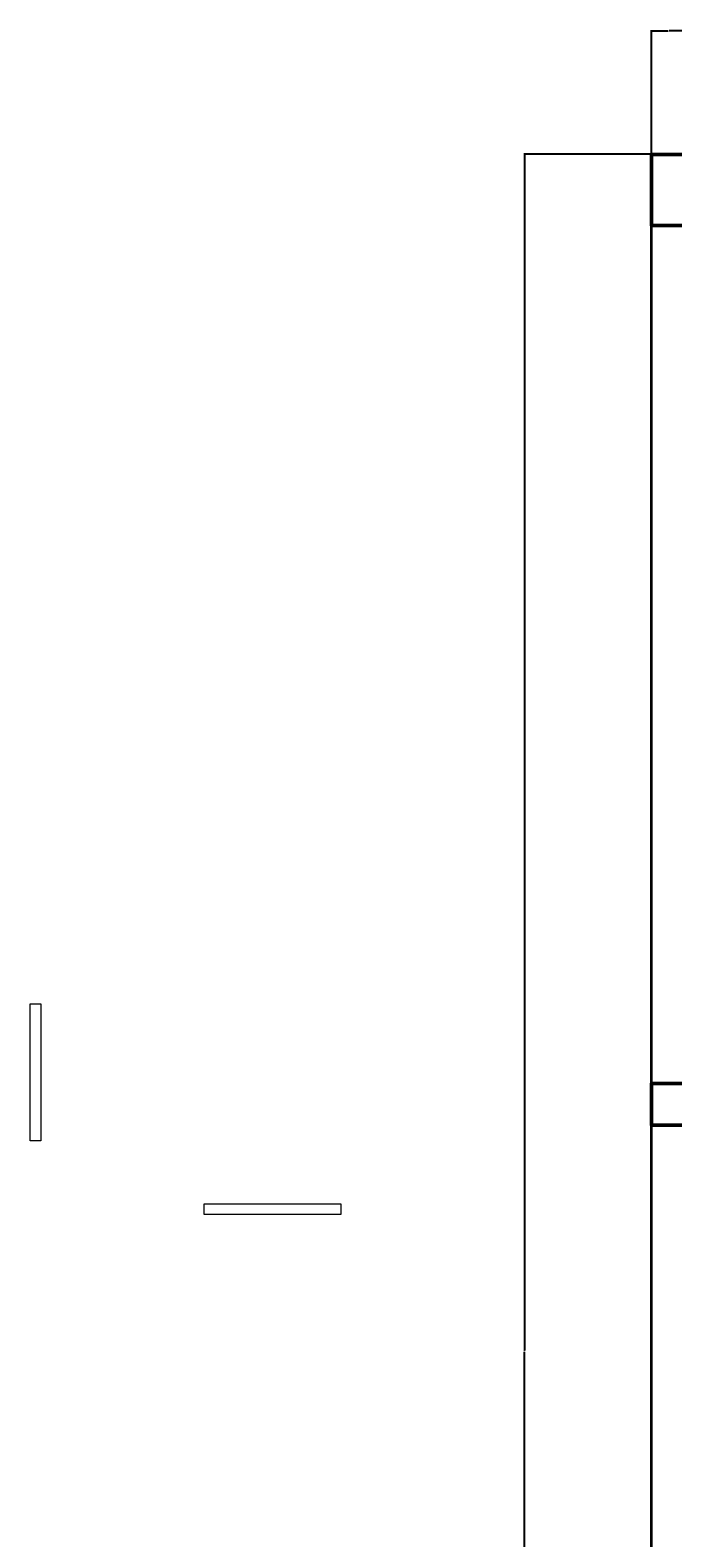
# Model space of a CAD drawing. Units: inches. Extents: x 50 to 2003, y -28 to 675.
# Tile 2 of 10: x 50 to 218, y 281 to 675. Entities that reach past the tile are written whole.
import ezdxf

# ---------------------------------------------------------------- set-up
doc = ezdxf.new("R2010")
doc.units = ezdxf.units.IN
for name, color, linetype, lineweight in [('A-ANNO-DIMS', 2, 'Continuous', 18), ('A-COLS', 1, 'Continuous', 50), ('A-DOOR', 4, 'Continuous', 18), ('A-WALL', 7, 'Continuous', 35)]:
    doc.layers.add(name, color=color, linetype=linetype, lineweight=lineweight)
doc.styles.get("Standard").update_dxf_attribs({"font": 'arial.ttf'})
doc.dimstyles.get("Standard").update_dxf_attribs({"dimtxt": 0.18, "dimasz": 0.18, "dimexe": 0.18, "dimexo": 0.0625, "dimgap": 0.09, "dimtad": 0, "dimtih": 1, "dimtoh": 1, "dimdec": 4, "dimzin": 0, "dimdsep": 46, "dimtxsty": 'Standard', "dimcen": 0.09, "dimadec": 0, "dimazin": 0, "dimtfac": 1, "dimtdec": 4, "dimtofl": 0, "dimtmove": 0, "dimatfit": 3, "dimfxl": 1, "dimtolj": 1, "dimtzin": 0, "dimarcsym": 0})

# ---------------------------------------------------------------- blocks, each defined once
blk = doc.blocks.new('DOOR-LEAF-36')
blk.add_lwpolyline([(35.71, 2.81), (35.71, 0), (0, 0), (0, 2.81)], close=True)
blk = doc.blocks.new('*D52')
at = {"layer": 'A-ANNO-DIMS', "color": 0, "lineweight": -2, "transparency": 16777216}
for p, q in [((211.91, 642.32), (178.66, 642.32)), ((178.84, 642.14), (178.84, 330.01)), ((178.84, 17.5), (178.84, 329.64)), ((211.91, 17.32), (178.66, 17.32))]:
    blk.add_line(p, q, dxfattribs=at)
at = {"layer": 'A-ANNO-DIMS', "color": 0, "transparency": 16777216}
for points in [[(178.81, 642.14), (178.87, 642.14), (178.84, 642.32)], [(178.81, 17.5), (178.87, 17.5), (178.84, 17.32)]]:
    blk.add_solid(points, dxfattribs=at)
at = {"layer": 'Defpoints', "color": 0, "transparency": 16777216}
for p in [(178.84, 642.32), (211.97, 642.32), (211.97, 17.32)]:
    blk.add_point(p, dxfattribs=at)
at = {"layer": 'A-ANNO-DIMS', "color": 0, "transparency": 16777216, "insert": (178.84, 329.82), "char_height": 0.18, "attachment_point": 5}
blk.add_mtext('\\A1;625', dxfattribs=at)
blk = doc.blocks.new('*D54')
at = {"layer": 'A-ANNO-DIMS', "color": 0, "lineweight": -2, "transparency": 16777216}
for p, q in [((211.97, 642.39), (211.97, 674.65)), ((212.15, 674.47), (216.32, 674.47)), ((220.79, 674.47), (216.62, 674.47)), ((220.97, 633.39), (220.97, 674.65))]:
    blk.add_line(p, q, dxfattribs=at)
at = {"layer": 'A-ANNO-DIMS', "color": 0, "transparency": 16777216}
for points in [[(212.15, 674.5), (212.15, 674.44), (211.97, 674.47)], [(220.79, 674.5), (220.79, 674.44), (220.97, 674.47)]]:
    blk.add_solid(points, dxfattribs=at)
at = {"layer": 'Defpoints', "color": 0, "transparency": 16777216}
for p in [(220.97, 674.47), (211.97, 642.32), (220.97, 633.32)]:
    blk.add_point(p, dxfattribs=at)
at = {"layer": 'A-ANNO-DIMS', "color": 0, "transparency": 16777216, "insert": (216.47, 674.47), "char_height": 0.18, "attachment_point": 5}
blk.add_mtext('\\A1;9', dxfattribs=at)

msp = doc.modelspace()

# ---------------------------------------------------------------- linework, layer by layer
at = {"layer": 'A-COLS'}
for points in [[(211.9898, 642.1898), (229.9336, 642.1898), (229.9336, 623.6596), (211.9898, 623.6596)], [(225.7742, 399.6502), (211.9886, 399.6502), (211.9886, 388.811), (225.7742, 388.811)]]:
    msp.add_lwpolyline(points, close=True, dxfattribs=at)
at = {"layer": 'A-WALL'}
for p, q in [((211.9711, 17.3232), (211.9711, 642.3232)), ((211.9711, 642.3232), (511.9711, 642.3232))]:
    msp.add_line(p, q, dxfattribs=at)

# ---------------------------------------------------------------- block references
at = {"layer": 'A-DOOR', "rotation": 269.9999999999998}
msp.add_blockref('DOOR-LEAF-36', (49.8071, 420.4647), dxfattribs=at)
at = {"layer": 'A-DOOR'}
msp.add_blockref('DOOR-LEAF-36', (95.1997, 365.492), dxfattribs=at)

# ---------------------------------------------------------------- dimensions: what is measured, and where the dimension line sits
at = {"layer": 'A-ANNO-DIMS'}
dim = msp.add_linear_dim(base=(220.9711, 674.4732), p1=(211.9711, 642.3232), p2=(220.9711, 633.3232), dimstyle='Standard', override={"dimdec": 0, "dimlfac": 1, "dimrnd": 0, "dimzin": 0, "dimdsep": 46, "dimlunit": 2}, dxfattribs=at)
dim.commit()
dim.dimension.update_dxf_attribs({"geometry": '*D54', "text_midpoint": (216.4711, 674.4732)})
dim = msp.add_linear_dim(base=(178.842, 642.3232), p1=(211.9711, 17.3232), p2=(211.9711, 642.3232), angle=90, dimstyle='Standard', override={"dimdec": 0, "dimlfac": 1, "dimrnd": 0, "dimzin": 0, "dimdsep": 46, "dimlunit": 2}, dxfattribs=at)
dim.commit()
dim.dimension.update_dxf_attribs({"geometry": '*D52', "text_midpoint": (178.842, 329.8232)})

doc.saveas('drawing.dxf')
